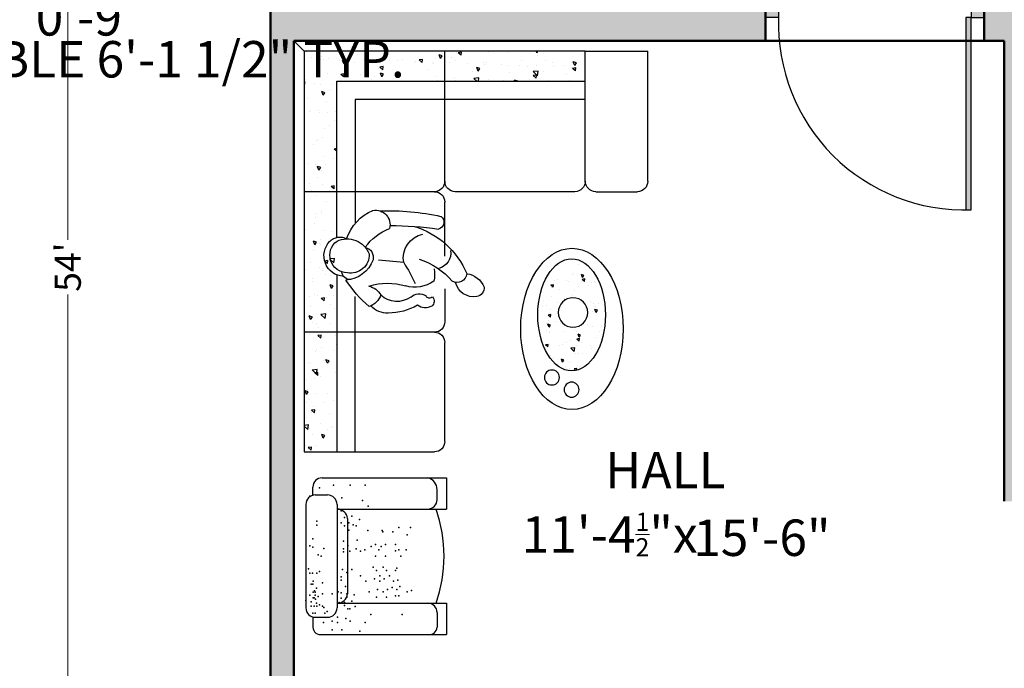
# Model space of a CAD drawing. Units: inches. Extents: x 4508 to 5907, y 877 to 1592.
# Tile 10 of 20: x 5203 to 5392, y 1174 to 1298. Entities that reach past the tile are written whole.
import ezdxf

# ---------------------------------------------------------------- set-up
doc = ezdxf.new("R2010")
doc.units = ezdxf.units.IN
doc.layers.get('DEFPOINTS').update_dxf_attribs({"color": 8})
for name, color, linetype, lineweight in [('A-ANNO-DIMS', 2, 'Continuous', 18), ('A-DOOR', 4, 'Continuous', 25), ('A-FURN', 24, 'Continuous', 18), ('A-WALL', 7, 'Continuous', 50), ('A-WALL-PATT', 8, 'Continuous', 13)]:
    doc.layers.add(name, color=color, linetype=linetype, lineweight=lineweight)
doc.layers.add('doors & windows', color=30, linetype='Continuous')
doc.layers.add('furniture', color=24, linetype='Continuous')
doc.styles.get("Standard").update_dxf_attribs({"font": 'arial.ttf'})
doc.dimstyles.new('details', dxfattribs={"dimtxt": 5, "dimasz": 2, "dimexe": 2, "dimexo": 3, "dimgap": 1, "dimtad": 0, "dimdec": 1, "dimzin": 0, "dimdsep": 46, "dimlunit": 4, "dimtxsty": 'Standard', "dimblk": 'ARCHTICK', "dimcen": 3, "dimclrd": 256, "dimclre": 256, "dimclrt": 256, "dimadec": 0, "dimazin": 0, "dimtfac": 0.5, "dimtdec": 1, "dimtofl": 0, "dimtmove": 0, "dimatfit": 3, "dimldrblk": 'CLOSEDBLANK', "dimfxl": 2, "dimtolj": 1, "dimtzin": 0, "dimlwd": -1, "dimlwe": -1, "dimarcsym": 0})
doc.dimstyles.new('text', dxfattribs={"dimtxt": 7, "dimasz": 0, "dimexe": 3, "dimexo": 3, "dimgap": 0, "dimtad": 1, "dimtih": 1, "dimtoh": 1, "dimzin": 3, "dimdsep": 46, "dimlunit": 4, "dimtxsty": 'Standard', "dimblk": 'CLOSEDBLANK', "dimcen": 3, "dimse1": 1, "dimse2": 1, "dimsd1": 1, "dimsd2": 1, "dimclrd": 256, "dimclre": 256, "dimclrt": 256, "dimadec": 0, "dimazin": 0, "dimtfac": 0.5, "dimtofl": 0, "dimtmove": 0, "dimatfit": 3, "dimfxl": 3, "dimtolj": 1, "dimtzin": 0, "dimlwd": -1, "dimlwe": -1, "dimarcsym": 0})

# ---------------------------------------------------------------- blocks, each defined once
blk = doc.blocks.new('_ArchTick')
at = {"color": 0, "linetype": 'ByBlock', "const_width": 0.15}
blk.add_lwpolyline([(-0.5, -0.5), (0.5, 0.5)], dxfattribs=at)
blk = doc.blocks.new('*D77')
at = {"layer": 'A-ANNO-DIMS', "color": 0, "transparency": 16777216}
for p, q in [((5201.49, 1574.7), (5213.97, 1574.7)), ((5211.97, 1574.7), (5211.97, 1255.95)), ((5211.97, 926.7), (5211.97, 1245.46)), ((5201.49, 926.7), (5213.97, 926.7))]:
    blk.add_line(p, q, dxfattribs=at)
at = {"layer": 'DEFPOINTS', "color": 0, "transparency": 16777216}
for p in [(5198.49, 1574.7), (5211.97, 1574.7), (5198.49, 926.7)]:
    blk.add_point(p, dxfattribs=at)
at = {"layer": 'A-ANNO-DIMS', "color": 0, "transparency": 16777216, "xscale": 2, "yscale": 2, "zscale": 2}
for p, rotation in [((5211.97, 1574.7), 90), ((5211.97, 926.7), 270)]:
    blk.add_blockref('_ArchTick', p, dxfattribs=dict(at, rotation=rotation))
at = {"layer": 'A-ANNO-DIMS', "color": 0, "transparency": 16777216, "insert": (5211.97, 1250.7), "char_height": 5, "attachment_point": 5, "rotation": 90}
blk.add_mtext("\\A1;54'", dxfattribs=at)
blk = doc.blocks.new('_ClosedBlank')
at = {"color": 0, "lineweight": -2}
for p, q in [((-1, 0.167), (0, 0)), ((-1, 0.167), (-1, -0.167)), ((0, 0), (-1, -0.167))]:
    blk.add_line(p, q, dxfattribs=at)
blk = doc.blocks.new('MAN')
at = {"layer": 'doors & windows'}
blk.add_line((1.3, -9.85), (0.89, -5.45), dxfattribs=at)
for centre, radius, start, end in [((0.1, 0.48), 3.6, 2.8928, 134.5528), ((-0.81, 1.3), 2.37, 132.7993, 210.1219), ((1.3, 0.05), 4.16, 155.2349, 248.5051), ((0, 0), 3.06, 359.7942, 144.0351), ((-0.36, -7.56), 8.07, 108.0153, 157.5724), ((-0.98, 0.55), 5.34, 289.2819, 356.6237), ((2.86, -0.44), 1.38, 352.7443, 87.7525), ((-8.99, -19.77), 24.04, 41.647, 56.3067), ((-0.1, -0.61), 3.22, 267.7788, 10.6507), ((4.14, -10.82), 9.46, 125.6851, 158.6987), ((0.38, -2.75), 1.79, 192.3382, 283.0231), ((-5.32, -4.92), 2.54, 170.002, 284.7527), ((15.87, -7.04), 10.97, 162.7002, 196.7262), ((8.59, -3.01), 3.29, 193.5598, 239.9446), ((5.83, -2.73), 3.32, 289.6374, 341.2911), ((6.12, -7.03), 4.01, 358.2671, 46.939), ((34.75, -7.19), 42.53, 177.9613, 192.4551), ((3.84, -8.67), 4.24, 325.4363, 41.8446), ((54.76, -7.35), 59.95, 180.1044, 188.2297), ((-0.78, -6.94), 10.91, 330.7562, 358.8997), ((0.5, -14.05), 4.27, 79.2575, 168.509), ((16.49, 13.41), 27.78, 236.8487, 245.427), ((-0.19, -11.81), 5.78, 325.2412, 16.1794), ((9.03, -7.36), 14.72, 197.1765, 246.7641), ((8.85, -12.54), 2.12, 136.0875, 215.1077), ((12.84, -8.62), 12.77, 197.9012, 229.3504), ((7.06, -13.61), 2.15, 328.4119, 38.6474), ((3.21, -8.72), 6.53, 262.8142, 281.931), ((6.8, -14.37), 0.689, 315.9836, 61.7947), ((8.05, -14.12), 1.05, 224.0636, 323.687), ((-5.78, -15.61), 1.25, 217.214, 345.0614), ((-0.4, -15.27), 2.81, 261.6005, 345.5998), ((3.09, -19.2), 1.68, 274.444, 31.8659), ((4.09, -22.01), 3.16, 349.15, 77.9716), ((6.99, -20.36), 3.8, 187.9766, 248.0432), ((5.75, -22.44), 1.45, 262.6631, 353.5986)]:
    blk.add_arc(centre, radius, start, end, dxfattribs=at)
blk = doc.blocks.new('sofa 3')
at = {"layer": 'furniture', "ltscale": 0.5}
h = blk.add_hatch(dxfattribs=at)
h.set_pattern_fill('AR-CONC', color=256, angle=90, style=0)
h.set_pattern_definition([(220, (1099.1507, -871.655), (0.627521, -7.172602), [0.75, -8.25]), (275, (1099.151, -871.655), (-7.52192, 1.387513), [0.6, -6.6]), (169.5486, (1099.203, -872.253), (-6.894395, -5.785094), [0.637402, -7.01142]), (223.8158, (1097.151, -871.655), (1.65519, -10.67241), [1.125, -12.375]), (173.3644, (1097.289, -872.544), (-9.74118, -9.34663), [0.9561, -10.51713]), (278.8158, (1097.151, -871.655), (-9.74119, -9.34662), [0.9, -9.9]), (249, (1097.6507, -872.655), (4.02619, -5.96907), [0.75, -8.25]), (304, (1097.651, -872.655), (-7.2515, -2.433153), [0.6, -6.6]), (198.5486, (1097.986, -873.1524), (-3.225305, -8.402226), [0.637402, -7.01142]), (232.5, (1099.1507, -871.655), (-3.3289385, -0.1215986), [0, -6.52, 0, -6.7, 0, -6.625]), (262.5, (1099.1507, -871.655), (-3.944117, -2.630695), [0, -3.82, 0, -6.37, 0, -2.525]), (302.5, (1099.1507, -869.425), (0.2255487, -5.3382244), [0, -2.5, 0, -7.8, 0, -10.35]), (312.5, (1099.1507, -868.425), (-1.00105, -5.831862), [0, -3.25, 0, -5.18, 0, -7.35])])
h.paths.add_polyline_path([(2, 56), (2, 79), (8.27, 79), (8.27, 56)])
edge = h.paths.add_edge_path()
edge.add_arc((9.44, 36.7), 1.54, 139.4115, 177.7525)
edge.add_arc((8.94, 33.52), 3.4, 107.8673, 234.0351)
edge.add_arc((8.88, 34.97), 4.62, 245.2349, 262.3616)
edge.add_line((8.27, 30.38), (8.27, 29))
edge.add_line((8.27, 29), (2, 29))
edge.add_line((2, 29), (2, 56))
edge.add_line((2, 56), (8.27, 56))
edge.add_line((8.27, 56), (8.27, 37.7))
h.paths.add_polyline_path([(8.27, 7.77), (29, 7.77), (29, 2), (2, 2), (2, 29), (8.27, 29)])
h.paths.add_polyline_path([(29, 2), (29, 7.77), (56, 7.77), (56, 2)])
at = {"layer": 'furniture'}
h = blk.add_hatch(dxfattribs=at)
h.set_pattern_fill('AR-CONC', color=256, scale=0.8, angle=90, style=0)
h.set_pattern_definition([(220, (892.888, -686.9864), (0.502017, -5.738081), [0.6, -6.6]), (275, (892.888, -686.9864), (-6.017537, 1.11001), [0.48, -5.28]), (169.5486, (892.93, -687.4646), (-5.515516, -4.628075), [0.509922, -5.609137]), (223.8158, (891.288, -686.9864), (1.32415, -8.53793), [0.9, -9.9]), (173.3644, (891.3985, -687.698), (-7.79294, -7.4773), [0.76488, -8.413704]), (278.8158, (891.288, -686.986), (-7.79295, -7.477296), [0.72, -7.92]), (249, (891.688, -687.7864), (3.220951, -4.775256), [0.6, -6.6]), (304, (891.688, -687.7864), (-5.8012, -1.946523), [0.48, -5.28]), (198.5486, (891.9566, -688.1844), (-2.580244, -6.72178), [0.509922, -5.609137]), (232.5, (892.8881, -686.9864), (-2.663151, -0.097279), [0, -5.216, 0, -5.36, 0, -5.3]), (262.5, (892.8881, -686.9864), (-3.155294, -2.104556), [0, -3.056, 0, -5.096, 0, -2.02]), (302.5, (892.8881, -685.2024), (0.180439, -4.2705795), [0, -2, 0, -6.24, 0, -8.28]), (312.5, (892.888, -684.4024), (-0.80084, -4.665489), [0, -2.6, 0, -4.144, 0, -5.88])])
edge = h.paths.add_edge_path()
edge.add_ellipse((53.37, 52.67), major_axis=(0, 10.76), ratio=0.60396, start_angle=0, end_angle=360, ccw=False)
h.paths.add_polyline_path([(56.46, 52.22, -1), (50.81, 52.22, -1)], flags=16)
for p, q in [((2, 2), (2, 79)), ((2, 79), (27, 79)), ((8.27, 44.99), (8.27, 79)), ((11.8, 79), (11.8, 49.12)), ((29, 77), (29, 58)), ((27, 56), (2, 56)), ((29, 47.65), (29, 54)), ((29, 41.41), (29, 31)), ((8.27, 37.77), (8.27, 7.77)), ((11.8, 11.29), (11.8, 35.08)), ((8.27, 29), (2, 29)), ((27, 29), (8.27, 29)), ((54, 29), (31, 29)), ((58, 29), (66, 29)), ((29, 27), (29, 2)), ((56, 27), (56, 2)), ((68, 27), (68, 2)), ((56, 11.29), (11.8, 11.29)), ((8.27, 7.77), (56, 7.77)), ((2, 2), (0, 0)), ((56, 2), (2, 2)), ((56, 2), (68, 2))]:
    blk.add_line(p, q, dxfattribs=at)
for centre, radius in [((53.36, 67.05), 1.44), ((49.58, 64.71), 1.44), ((53.63, 52.22), 2.83)]:
    blk.add_circle(centre, radius, dxfattribs=at)
for centre, start, end in [((27, 77), 0, 90), ((27, 58), 270, 0), ((27, 54), 0, 90), ((27, 31), 270, 0), ((27, 27), 0, 90), ((31, 27), 90, 180), ((54, 27), 0, 90), ((58, 27), 90, 180), ((66, 27), 0, 90)]:
    blk.add_arc(centre, 2, start, end, dxfattribs=at)
at = {"layer": 'furniture', "extrusion": (0, 0, -1)}
for centre, major_axis, ratio in [((53.43, 55.37), (0, 15.49), 0.635514), ((53.37, 52.67), (0, 10.76), 0.60396)]:
    blk.add_ellipse(centre, major_axis=major_axis, ratio=ratio, dxfattribs=at)
at = {"xscale": 1.1, "yscale": 1.1, "zscale": 1.1, "rotation": 90}
blk.add_blockref('MAN', (10.27, 41.21), dxfattribs=at)
blk = doc.blocks.new('MD')
at = {"layer": 'doors & windows'}
h = blk.add_hatch(dxfattribs=at)
h.set_pattern_fill('DOTS', color=256, scale=2, style=0)
h.set_pattern_definition([(180, (0, -4), (-0.0625, 0.125), [0, -0.125])])
h.paths.add_polyline_path([(2.5, 37), (3.5, 37), (3.5, 0), (2.5, 0)])
h = blk.add_hatch(dxfattribs=at)
h.set_pattern_fill('DOTS', color=256, scale=2, style=0)
h.set_pattern_definition([(0, (0, -0.5), (0.0625, 0.125), [0, -0.125])])
h.paths.add_polyline_path([(42, -4.5), (42, 0), (39.5, 0), (39.5, -1.5), (39, -1.5), (39, -3.75), (39.25, -3.75, 0.403966), (39.75, -4.25), (39.75, -4.5)])
h.paths.add_polyline_path([(0, -4.5), (2.25, -4.5), (2.25, -4.25, 0.403966), (2.75, -3.75), (3, -3.75), (3, -1.5), (2.5, -1.5), (2.5, 0), (0, 0)])
for p, q in [((0, 0), (0, -4.5)), ((42, 0), (42, -4.5))]:
    blk.add_line(p, q)
blk.add_line((0, -4.5), (2.25, -4.5), dxfattribs=at)
blk.add_lwpolyline([(3.5, 0), (3.5, 37), (2.5, 37), (2.5, 0)], close=True, dxfattribs=at)
for points in [[(3, -3.75), (3, -1.5), (2.5, -1.5), (2.5, 0), (0, 0)], [(39, -3.75), (39, -1.5), (39.5, -1.5), (39.5, 0), (42, 0)], [(42, -4.5), (39.75, -4.5)]]:
    blk.add_lwpolyline(points, dxfattribs=at)
for points in [[(2.25, -4.5), (2.25, -4.25, 0.403966), (2.75, -3.75), (3, -3.75)], [(39.75, -4.5), (39.75, -4.25, -0.403966), (39.25, -3.75), (39, -3.75)]]:
    blk.add_lwpolyline(points, format="xyb", dxfattribs=at)
at = {"layer": 'doors & windows', "ltscale": 6}
blk.add_arc((3.73, 1.23), 35.79, 358.0281, 91.9719, dxfattribs=at)
at = {"layer": 'doors & windows'}
blk.add_point((21, -2.75), dxfattribs=at)
blk = doc.blocks.new('sofa')
at = {"layer": 'furniture'}
for p, q in [((1.33, 11.75), (1.33, 13.25)), ((3.13, 15.05), (27, 15.05)), ((27, 15.05), (27, 9.05)), ((1.8, 11.75), (4.13, 11.75)), ((25.2, 10.85), (25.2, 12.75)), ((0, 9.95), (0, -9.95)), ((6, 9.95), (6, -9.95)), ((6, 9.05), (27, 9.05)), ((8, 7.25), (8, -7.25)), ((8, 4.04), (8, 3.89)), ((6.03, -9.05), (27, -9.05)), ((27, -9.05), (27, -15.05)), ((25.2, -10.85), (25.2, -13.65)), ((1.33, -11.75), (1.33, -13.65)), ((1.8, -11.75), (4.13, -11.75)), ((3.13, -15.05), (27, -15.05))]:
    blk.add_line(p, q, dxfattribs=at)
for centre, radius, start, end in [((3.13, 13.25), 1.8, 90, 180), ((22.91, 12.82), 2.29, 358.3453, 77.7487), ((1.8, 9.95), 1.8, 90, 180), ((1.8, 9.95), 1.8, 90, 180), ((4.14, 9.89), 1.86, 1.747, 90.2901), ((4.14, 9.89), 1.86, 1.747, 90.2901), ((23.4, 10.85), 1.8, 270, 0), ((5.91, 6.93), 2.12, 8.589, 87.4366), ((-0.79, 0), 27.33, 340.6621, 19.3379), ((5.96, -6.99), 2.06, 272.0036, 352.7589), ((23.4, -10.85), 1.8, 0, 90), ((1.8, -9.95), 1.8, 180, 270), ((4.14, -9.89), 1.86, 269.7099, 358.253), ((2.83, -13.59), 1.5, 182.4941, 281.7559), ((23.7, -13.59), 1.5, 258.2441, 357.5059)]:
    blk.add_arc(centre, radius, start, end, dxfattribs=at)
for p in [(5.3, 13.66), (8.48, 13.66), (11.4, 13.66), (0.72, 11.51), (2.64, 13.13), (6.89, 11.2), (10.87, 10.67), (11.93, 9.61), (6.8, 8.68), (8.85, 7.66), (2.09, 5.95), (2.11, 6.75), (6.8, 6.43), (7.42, 7.45), (7.42, 5.82), (8.24, 6.43), (9.05, 6.02), (9.67, 5.82), (10.28, 7.04), (8.24, 5), (11.92, 4.9), (14.64, 4.9), (14.78, 4.7), (16.69, 4.7), (17.83, 5.52), (19.47, 4.09), (20.08, 5.52), (0.72, 1.97), (1.32, 3.3), (7.21, 2.86), (8.03, 2.04), (9.87, 3.06), (13.35, 2.21), (15.26, 2.21), (17.21, 2.25), (1.3, 1.71), (2.38, 0.24), (3.44, 1.44), (7.21, 1.39), (7.21, 0.82), (8.44, 0.98), (9.67, 1.43), (10.49, 0.98), (11.31, 1.19), (12.53, 1.84), (13.35, 0.01), (14.03, 1.19), (14.44, 1.84), (15.26, 0.01), (17.24, 1.02), (17.85, 1.19), (19.26, 1.19), (2.91, -0.01), (18.24, -0.03), (0.5, -2.45), (0.72, -3.25), (1.26, -3.25), (2.11, -3.25), (2.64, -2.98), (7.01, -2.55), (7.83, -3.16), (8.85, -2.55), (10.49, -3.77), (12.94, -2.14), (13.56, -2.75), (14.17, -3.77), (14.85, -2.14), (15.46, -2.75), (16.07, -3.77), (17.21, -2.75), (17.44, -2.34), (1.03, -5.36), (1.32, -5.36), (1.36, -4.83), (3.17, -5.1), (6.8, -3.98), (6.8, -4.59), (11.51, -4.79), (13.15, -4.38), (14.23, -4.79), (15.05, -4.38), (16.8, -4.79), (17.65, -4.59), (0.77, -7.48), (1.36, -6.95), (1.62, -6.69), (1.79, -6.95), (1.79, -7.48), (2.05, -6.16), (3.17, -7.22), (5.03, -7.22), (6.19, -6.84), (6.8, -7.04), (7.62, -5.82), (7.83, -7.25), (9.26, -7.45), (12.12, -6.84), (13.76, -6.43), (14.85, -6.84), (15.66, -6.43), (16.6, -6.02), (17.44, -6.43), (18.06, -5.82), (19.47, -6.84), (20.28, -6.63), (-0.03, -8.54), (1.03, -8.81), (1.36, -8.01), (1.56, -8.01), (1.85, -8.28), (2.05, -9.07), (2.38, -7.75), (2.64, -9.34), (6.39, -8.88), (6.8, -8.06), (7.42, -8.88), (7.83, -7.86), (8.85, -8.68), (13.56, -7.86), (15.46, -7.86), (17.24, -7.65), (17.83, -7.65), (0.99, -9.6), (1.3, -10.93), (1.58, -9.6), (1.79, -10.93), (2.09, -9.6), (3.17, -9.6), (3.44, -9.87), (3.64, -10.93), (4.09, -10.66), (7.42, -9.49), (8.03, -10.11), (8.44, -10.11), (9.46, -9.7), (12.46, -11.19), (18.51, -11.19), (3.38, -12.78), (5.03, -12.52), (6.09, -11.72), (6.09, -12.78), (7.69, -11.99), (8.48, -12.52), (11.4, -12.78), (5.03, -14.17), (6.89, -14.17), (10.34, -14.44)]:
    blk.add_point(p, dxfattribs=at)
blk = doc.blocks.new('*D98')
at = {"layer": 'DEFPOINTS', "color": 0, "transparency": 16777216}
for p in [(5255.4, 1205.15), (5391.9, 1205.7), (5255.4, 1203.74)]:
    blk.add_point(p, dxfattribs=at)
at = {"layer": 'A-ANNO-DIMS', "color": 0, "transparency": 16777216, "insert": (5316.09, 1205.15), "char_height": 7, "attachment_point": 5}
blk.add_mtext('\\A1;          HALL\\P11\'-4{\\H0.5x;\\S1/2;}"x', dxfattribs=at)
blk = doc.blocks.new('*D99')
at = {"layer": 'DEFPOINTS', "color": 0, "transparency": 16777216}
for p in [(5336.4, 1294.2), (5345.32, 1294.2), (5334.11, 1108.2)]:
    blk.add_point(p, dxfattribs=at)
at = {"layer": 'A-ANNO-DIMS', "color": 0, "transparency": 16777216, "insert": (5345.32, 1198.7), "char_height": 7, "attachment_point": 5}
blk.add_mtext('\\A1;15\'-6"', dxfattribs=at)
blk = doc.blocks.new('*D172')
at = {"layer": 'DEFPOINTS', "color": 0, "transparency": 16777216}
for p in [(5076.25, 1287.03), (5076.25, 1276.01), (5149.75, 1276.01)]:
    blk.add_point(p, dxfattribs=at)
at = {"layer": 'A-ANNO-DIMS', "transparency": 16777216, "insert": (5214.38, 1290.65), "char_height": 7, "attachment_point": 5}
blk.add_mtext('\\A1;DINING TABLE 6\'-1 1/2" TYP.', dxfattribs=at)
blk = doc.blocks.new('*D188')
at = {"layer": 'DEFPOINTS', "color": 0, "transparency": 16777216}
for p in [(5259.90304, 1303.203772), (5216.35304, 1294.203772), (5255.40304, 1294.203772)]:
    blk.add_point(p, dxfattribs=at)
at = {"layer": 'A-ANNO-DIMS', "transparency": 16777216, "insert": (5216.35304, 1298.703772), "char_height": 7, "attachment_point": 5}
blk.add_mtext('\\A1;0\'-9"', dxfattribs=at)

msp = doc.modelspace()

# ---------------------------------------------------------------- hatches: boundary and pattern name
at = {"layer": 'A-WALL-PATT'}
h = msp.add_hatch(color=256, dxfattribs=at)
h.dxf.hatch_style = 1
h.paths.add_polyline_path([(5529.903, 1303.204), (5388.02, 1303.204), (5388.02, 1294.204), (5391.903, 1294.204), (5391.903, 1205.704), (5396.403, 1205.704), (5396.403, 1294.204), (5489.403, 1294.204), (5489.403, 1256.139), (5493.903, 1256.139), (5493.903, 1294.204), (5529.903, 1294.204)], flags=17)
h.paths.add_polyline_path([(5346.02, 1303.204), (5322.903, 1303.204), (5322.903, 1321.388), (5313.903, 1321.388), (5313.903, 1303.204), (5259.903, 1303.204), (5259.903, 1381.204), (5313.903, 1381.204), (5313.903, 1359.674), (5322.903, 1359.674), (5322.903, 1381.204), (5338.979, 1381.204), (5338.979, 1390.204), (5331.903, 1390.204), (5331.903, 1442.704), (5255.403, 1442.704), (5255.403, 1570.204), (5387.403, 1570.204), (5387.403, 1541.271), (5391.903, 1541.271), (5391.903, 1570.204), (5483.403, 1570.204), (5483.403, 1498.204), (5391.903, 1498.204), (5391.903, 1509.559), (5387.403, 1509.559), (5387.403, 1390.204), (5380.979, 1390.204), (5380.979, 1381.204), (5387.403, 1381.204), (5529.903, 1381.204), (5529.903, 1498.204), (5487.903, 1498.204), (5487.903, 1570.204), (5529.903, 1570.204), (5529.903, 1574.704), (5250.903, 1574.704), (5250.903, 991.204), (5310.903, 991.204), (5310.903, 926.704), (5529.903, 926.704), (5529.903, 1210.204), (5525.403, 1210.204), (5525.403, 1103.704), (5499.903, 1103.704), (5499.903, 1210.204), (5493.903, 1210.204), (5493.903, 1256.139), (5489.403, 1256.139), (5489.403, 1210.204), (5461.584, 1210.204), (5461.584, 1205.704), (5495.403, 1205.704), (5495.403, 1103.704), (5436.903, 1103.704), (5436.903, 1051.204), (5391.954, 1051.204), (5391.954, 1103.03), (5391.954, 1107.53), (5255.403, 1108.204), (5255.403, 1294.204), (5346.02, 1294.204)])
h.paths.add_polyline_path([(5255.403, 1390.204), (5255.403, 1398.204), (5255.403, 1438.204), (5257.903, 1438.204), (5258.903, 1438.204), (5327.403, 1438.204), (5327.403, 1390.204), (5325.903, 1390.204)], flags=16)
h.paths.add_polyline_path([(5288.757, 1390.704), (5288.757, 1390.204), (5292.173, 1390.204), (5292.173, 1390.704)], flags=0)
h.paths.add_polyline_path([(5289.965, 1391.606), (5289.965, 1396.645), (5289.903, 1396.645), (5289.903, 1397.319), (5288.849, 1398.862), (5288.849, 1398.8), (5288.983, 1398.748), (5288.983, 1399.204), (5289.091, 1399.204), (5292.081, 1399.204), (5292.081, 1398.665), (5291.946, 1398.665), (5291.027, 1397.319), (5291.027, 1396.645), (5290.965, 1396.645), (5290.965, 1391.606)], flags=0)
h.paths.add_polyline_path([(5288.849, 1399.069, 2.6374395), (5289.056, 1398.835), (5289.117, 1399.087, 0.9346155)], flags=0)
h.paths.add_polyline_path([(5290.061, 1398.665), (5290.061, 1399.204), (5290.038, 1398.975)], flags=0)
h.paths.add_polyline_path([(5291.946, 1398.934, -1), (5291.946, 1398.665)], flags=0)
h.paths.add_polyline_path([(5289.414, 1398.967), (5289.414, 1399.204), (5289.63, 1399.204), (5289.63, 1398.363), (5290.051, 1397.184), (5290.76, 1397.184), (5290.869, 1398.665), (5290.869, 1399.204), (5290.815, 1398.665), (5290.815, 1399.204), (5291.462, 1399.204), (5291.462, 1398.816), (5290.879, 1397.184), (5290.051, 1397.184)], flags=0)
h.paths.add_polyline_path([(5273.903, 1392.056), (5269.591, 1392.056, 0.0901028), (5265.544, 1392.842), (5265.511, 1392.034, -0.3516542), (5265.903, 1391.546, -1), (5264.903, 1391.546, -0.3042165), (5265.213, 1392.008), (5265.167, 1392.84, 0.0880132), (5261.215, 1392.056), (5256.903, 1392.056), (5256.903, 1398.704, -0.4142136), (5259.403, 1401.204), (5271.403, 1401.204, -0.4142136), (5273.903, 1398.704)], flags=0)
h.paths.add_polyline_path([(5263.726, 1395.073, -1), (5267.08, 1395.073, -1)], flags=0)
h.paths.add_polyline_path([(5264.434, 1395.073, -0.695521), (5265.153, 1395.073, -1.1408699), (5265.403, 1395.585, -0.7522125), (5265.403, 1396.25, 0.3674806)], flags=0)
h.paths.add_polyline_path([(5265.153, 1394.399, -1), (5265.653, 1394.399, -1)], flags=0)
h.paths.add_polyline_path([(5265.905, 1395.077, -1), (5266.405, 1395.077, -1)], flags=0)
h.paths.add_polyline_path([(5307.994, 1403.113, -1), (5307.994, 1417.295), (5318.794, 1417.295, -0.4142136), (5319.794, 1416.295), (5320.794, 1416.295, -0.4142136), (5321.794, 1417.295), (5324.903, 1417.295, -0.4142136), (5325.903, 1416.295), (5325.903, 1404.113, -0.4142136), (5324.903, 1403.113), (5321.794, 1403.113, -0.4142136), (5320.794, 1404.113), (5319.794, 1404.113, -0.4142136), (5318.794, 1403.113)], flags=0)
h.paths.add_polyline_path([(5307.836, 1405.113, -1), (5307.836, 1415.295), (5315.591, 1415.295, -0.4142136), (5317.532, 1413.353), (5317.532, 1407.054, -0.4142136), (5315.591, 1405.113)], flags=0)
h.paths.add_polyline_path([(5312.032, 1408.204, -1), (5312.032, 1412.204), (5315.032, 1412.204, -0.4142136), (5316.032, 1411.204), (5316.032, 1409.204, -0.4142136), (5315.032, 1408.204)], flags=0)
h.paths.add_polyline_path([(5391.903, 1385.704), (5391.903, 1493.704), (5525.403, 1493.704), (5525.403, 1385.704)], flags=16)
h.paths.add_polyline_path([(5422.641, 1390.704), (5422.641, 1465.704, -0.9426302), (5422.641, 1467.704), (5494.547, 1467.704, -1), (5494.665, 1465.704), (5494.665, 1390.704, -0.9426302), (5494.665, 1388.704), (5422.759, 1388.704, -1)], flags=0)
h.paths.add_polyline_path([(5427.52, 1395.749, -0.0238564), (5427.614, 1403.949, 0.0884332), (5427.476, 1405.056, 0.0506693), (5427.273, 1405.463, -0.8716827), (5427.713, 1405.835, 0.0268855), (5431.815, 1405.361, 0.0306964), (5436.289, 1405.361, -0.0263641), (5445.798, 1405.259, 0.075811), (5450.408, 1405.53, 0.0687062), (5454.457, 1405.903, -1.0086747), (5454.781, 1405.482, 0.0692081), (5454.389, 1400.959, -0.0519468), (5454.356, 1394.996, 0.1195012), (5454.627, 1392.895, 0.0143508), (5454.796, 1392.489, -0.6962059), (5454.42, 1392.118, 0.1574808), (5448.747, 1392.794, -0.025536), (5432.749, 1392.774, 0.0920085), (5427.781, 1392.048, -0.9384848), (5427.137, 1392.455, 0.0063894), (5427.314, 1392.79, 0.0472995)], flags=0)
h.paths.add_polyline_path([(5426.125, 1411.372, 0.0617649), (5428.641, 1412.201), (5428.641, 1465.704), (5488.665, 1465.704), (5488.665, 1412.363, 0.2363822), (5467.6, 1412.052, -0.2252042)], flags=0)
h.paths.add_polyline_path([(5391.903, 1490.204), (5391.903, 1491.204), (5422.903, 1491.204), (5422.903, 1490.204)], flags=0)
h.paths.add_polyline_path([(5462.545, 1392.771, 0.1270318), (5462.866, 1394.996, -0.0519468), (5462.832, 1400.959, 0.0692081), (5462.441, 1405.482, -1.0086747), (5462.765, 1405.903, 0.0857004), (5471.424, 1405.259, -0.0263641), (5480.932, 1405.361, 0.0306964), (5485.407, 1405.361, 0.0268855), (5489.509, 1405.835, -0.8716827), (5489.949, 1405.463, 0.0506693), (5489.746, 1405.056, 0.0884332), (5489.608, 1403.949, -0.0238564), (5489.702, 1395.749, 0.0472995), (5489.908, 1392.79, 0.0063894), (5490.085, 1392.455, -0.9384848), (5489.441, 1392.048, 0.0920085), (5484.473, 1392.774, -0.025536), (5468.475, 1392.794, 0.1574808), (5462.802, 1392.118, -0.6962059), (5462.426, 1392.489, 0.0100173), (5462.546, 1392.771)], flags=0)
h.paths.add_polyline_path([(5387.454, 1103.03), (5387.454, 1100.53), (5387.454, 1099.53), (5387.454, 995.03), (5387.454, 991.204), (5391.954, 991.204), (5391.954, 1046.704), (5525.403, 1046.704), (5525.403, 931.182), (5391.954, 930.53), (5391.954, 960.53), (5387.454, 960.53), (5387.454, 930.53), (5315.403, 930.53), (5315.403, 991.204), (5323.403, 991.204), (5387.454, 991.204), (5387.454, 995.03), (5255.403, 995.704), (5255.403, 1103.704)], flags=16)
h.paths.add_polyline_path([(5379.264, 1062.889), (5379.264, 1060.156), (5385.764, 1061.889, -0.4526903), (5385.764, 1059.889), (5379.264, 1059.889), (5379.264, 1055.156), (5385.764, 1056.889, -0.4526903), (5385.764, 1054.889), (5379.264, 1054.889), (5379.264, 1050.156), (5385.764, 1051.889, -0.4526903), (5385.764, 1049.889), (5379.264, 1049.889), (5379.264, 1010.156), (5385.764, 1011.889, -0.4526903), (5385.764, 1009.889), (5379.264, 1009.889), (5379.264, 1005.156), (5385.764, 1006.889, -0.4526903), (5385.764, 1004.889), (5379.264, 1004.889), (5379.264, 1000.156), (5385.764, 1001.889, -0.4526903), (5385.764, 999.889), (5378.264, 999.889), (5370.764, 997.889, -0.6674863), (5370.764, 999.889), (5377.264, 999.889), (5377.264, 1004.623), (5370.764, 1002.889, -0.6674863), (5370.764, 1004.889), (5377.264, 1004.889), (5377.264, 1009.623), (5370.764, 1007.889, -0.6674863), (5370.764, 1009.889), (5377.264, 1009.889), (5377.264, 1049.623), (5370.764, 1047.889, -0.6674863), (5370.764, 1049.889), (5377.264, 1049.889), (5377.264, 1054.623), (5370.764, 1052.889, -0.6674863), (5370.764, 1054.889), (5377.264, 1054.889), (5377.264, 1059.623), (5370.764, 1057.889, -0.6674863), (5370.764, 1059.889), (5377.264, 1059.889), (5377.264, 1062.889)], flags=0)
h.paths.add_polyline_path([(5287.641, 1000.704), (5359.665, 1000.704), (5359.665, 1018.212, 0.3202856), (5332.6, 1022.052, -0.246494), (5287.641, 1023.128)], flags=0)
h.paths.add_polyline_path([(5359.547, 1077.704, -1), (5359.665, 1075.704), (5353.665, 1075.704), (5353.665, 1063.704), (5293.641, 1063.704), (5293.641, 1075.704), (5287.759, 1075.704, -1), (5287.641, 1077.704)], flags=0)
h.paths.add_polyline_path([(5441.403, 1099.204), (5525.403, 1099.204), (5525.403, 1051.204), (5441.403, 1051.204), (5441.403, 1059.204)], flags=16)
h.paths.add_polyline_path([(5441.403, 1096.704), (5466.403, 1096.704), (5466.403, 1095.704), (5441.403, 1095.704)], flags=0)
h.paths.add_polyline_path([(5445.403, 1062.204), (5457.403, 1062.204, -0.4142136), (5459.903, 1059.704), (5459.903, 1053.056), (5455.591, 1053.056, 0.0901028), (5451.544, 1053.842), (5451.511, 1053.034, -0.3516542), (5451.903, 1052.546, -1), (5450.903, 1052.546, -0.3042165), (5451.213, 1053.008), (5451.167, 1053.84, 0.0880132), (5447.215, 1053.056), (5442.903, 1053.056), (5442.903, 1059.704, -0.4142136)], flags=0)
h.paths.add_polyline_path([(5453.08, 1056.073, -1), (5449.726, 1056.073, -1)], flags=0)
h.paths.add_polyline_path([(5292.713, 1015.835, 0.0268855), (5296.815, 1015.361, 0.0306964), (5301.289, 1015.361, -0.0263641), (5310.798, 1015.259, 0.075811), (5315.408, 1015.53, 0.0687062), (5319.457, 1015.903, -1.0086747), (5319.781, 1015.482, 0.0692081), (5319.389, 1010.959, -0.0519468), (5319.356, 1004.996, 0.1195012), (5319.627, 1002.895, 0.0143508), (5319.796, 1002.489, -0.6962059), (5319.42, 1002.118, 0.1574808), (5313.747, 1002.794, -0.025536), (5297.749, 1002.774, 0.0920085), (5292.781, 1002.048, -0.9384848), (5292.137, 1002.455, 0.0063894), (5292.314, 1002.79, 0.0472995), (5292.52, 1005.749, -0.0238564), (5292.614, 1013.949, 0.0884332), (5292.476, 1015.056, 0.0506693), (5292.273, 1015.463, -0.8716827)], flags=0)
h.paths.add_polyline_path([(5450.434, 1056.073, -0.695521), (5451.153, 1056.073, -1.1408699), (5451.403, 1056.585, -0.7522125), (5451.403, 1057.25, 0.3674806)], flags=0)
h.paths.add_polyline_path([(5327.765, 1015.903, 0.0857004), (5336.424, 1015.259, -0.0263641), (5345.932, 1015.361, 0.0306964), (5350.407, 1015.361, 0.0268855), (5354.509, 1015.835, -0.8716827), (5354.949, 1015.463, 0.0506693), (5354.746, 1015.056, 0.0884332), (5354.608, 1013.949, -0.0238564), (5354.702, 1005.749, 0.0472995), (5354.908, 1002.79, 0.0063894), (5355.085, 1002.455, -0.9384848), (5354.441, 1002.048, 0.0920085), (5349.473, 1002.774, -0.025536), (5333.475, 1002.794, 0.1574808), (5327.802, 1002.118, -0.6962059), (5327.426, 1002.489, 0.0100173), (5327.546, 1002.771), (5327.545, 1002.771, 0.1270318), (5327.866, 1004.996, -0.0519468), (5327.832, 1010.959, 0.0692081), (5327.441, 1015.482, -1.0086747)], flags=0)
h.paths.add_polyline_path([(5452.405, 1056.077, -1), (5451.905, 1056.077, -1)], flags=0)
h.paths.add_polyline_path([(5451.653, 1055.399, -1), (5451.153, 1055.399, -1)], flags=0)
h.paths.add_polyline_path([(5472.958, 1051.704), (5472.958, 1051.204), (5476.374, 1051.204), (5476.374, 1051.704)], flags=0)
h.paths.add_polyline_path([(5476.282, 1060.204), (5476.282, 1059.665), (5476.147, 1059.665), (5475.228, 1058.319), (5475.228, 1057.645), (5475.166, 1052.606), (5474.166, 1052.606), (5474.166, 1057.645), (5474.104, 1057.645), (5474.104, 1058.319), (5473.05, 1059.862), (5473.05, 1059.8), (5473.184, 1059.748), (5473.184, 1060.204), (5473.292, 1060.204)], flags=0)
h.paths.add_polyline_path([(5473.05, 1060.069, 2.6374395), (5473.257, 1059.835), (5473.318, 1060.087, 0.9346155)], flags=0)
h.paths.add_polyline_path([(5473.831, 1060.204), (5473.831, 1059.363), (5474.252, 1058.184), (5474.371, 1058.184), (5474.262, 1059.665), (5474.262, 1060.204)], flags=0)
h.paths.add_polyline_path([(5475.501, 1060.204), (5475.501, 1059.363), (5475.555, 1059.514), (5475.555, 1060.204)], flags=0)
h.paths.add_polyline_path([(5474.855, 1060.204), (5474.908, 1060.127), (5474.908, 1060.204), (5474.855, 1059.665)], flags=0)
h.paths.add_polyline_path([(5476.147, 1059.934, -1), (5476.147, 1059.665)], flags=0)
h.paths.add_polyline_path([(5474.693, 1060.204), (5475.178, 1059.511), (5475.178, 1060.204), (5475.285, 1059.934), (5475.285, 1060.204), (5475.178, 1059.665), (5475.178, 1060.204), (5475.07, 1059.665), (5475.07, 1060.204), (5474.962, 1059.665), (5474.962, 1060.204), (5474.693, 1059.306)], flags=0)
h.paths.add_polyline_path([(5474.747, 1060.204), (5474.37, 1059.45), (5474.37, 1060.204), (5474.424, 1060.096), (5474.424, 1060.204), (5474.747, 1059.665)], flags=0)
h.paths.add_polyline_path([(5476.04, 1059.665), (5476.04, 1060.204), (5476.094, 1059.665), (5476.094, 1060.204)], flags=0)
h.paths.add_polyline_path([(5505.994, 1082.295), (5516.794, 1082.295, -0.4142136), (5517.794, 1081.295), (5518.794, 1081.295, -0.4142136), (5519.794, 1082.295), (5522.903, 1082.295, -0.4142136), (5523.903, 1081.295), (5523.903, 1069.113, -0.4142136), (5522.903, 1068.113), (5519.794, 1068.113, -0.4142136), (5518.794, 1069.113), (5517.794, 1069.113, -0.4142136), (5516.794, 1068.113), (5505.994, 1068.113, -1)], flags=0)
h.paths.add_polyline_path([(5505.836, 1080.295), (5513.591, 1080.295, -0.4142136), (5515.532, 1078.353), (5515.532, 1072.054, -0.4142136), (5513.591, 1070.113), (5505.836, 1070.113, -1)], flags=0)
h.paths.add_polyline_path([(5520.403, 963.695), (5520.403, 1035.72), (5502.895, 1035.72, 0.3202856), (5499.055, 1008.654, -0.246494), (5497.978, 963.695)], flags=0)
h.paths.add_polyline_path([(5445.403, 1035.72), (5445.403, 1029.72), (5457.403, 1029.72), (5457.403, 969.695), (5445.403, 969.695), (5445.403, 963.814, -1), (5443.403, 963.695), (5443.403, 1035.602, -1)], flags=0)
h.paths.add_polyline_path([(5510.032, 1077.204), (5513.032, 1077.204, -0.4142136), (5514.032, 1076.204), (5514.032, 1074.204, -0.4142136), (5513.032, 1073.204), (5510.032, 1073.204, -1)], flags=0)
h.paths.add_polyline_path([(5317.255, 989.704), (5323.903, 989.704, -0.4142136), (5326.403, 987.204), (5326.403, 975.204, -0.4142136), (5323.903, 972.704), (5317.255, 972.704), (5317.255, 977.016, 0.0901028), (5318.041, 981.063), (5317.233, 981.096, -0.8964437), (5316.245, 981.204, -0.8220123), (5317.207, 981.394), (5318.04, 981.44, 0.0880132), (5317.255, 985.392)], flags=0)
h.paths.add_polyline_path([(5321.949, 981.204, -1), (5318.594, 981.204, -1)], flags=0)
h.paths.add_polyline_path([(5362.454, 988.03), (5387.454, 988.03), (5387.454, 990.53), (5391.954, 990.53), (5391.704, 988.289, -0.4090807), (5391.204, 987.78), (5391.204, 987.53), (5388.954, 987.53), (5388.954, 988.03), (5387.454, 988.03), (5387.454, 987.03), (5362.474, 987.03, 0.4025427), (5387.454, 963.03), (5388.954, 963.03), (5388.954, 963.53), (5391.195, 963.28, -0.4142136), (5391.704, 962.771), (5391.954, 960.53), (5391.954, 962.78), (5391.704, 962.78, 0.4090807), (5391.195, 963.28), (5388.954, 963.53), (5388.954, 963.03), (5387.454, 963.03, -0.4025427), (5362.474, 987.03), (5362.454, 987.03)], flags=0)
h.paths.add_polyline_path([(5321.285, 981.204, -0.6555366), (5320.522, 981.204, -1.1195284), (5320.275, 980.701, -1.3500746), (5320.279, 980.026, 0.3749463)], flags=0)
h.paths.add_polyline_path([(5320.022, 981.923, -1), (5320.522, 981.923, -1)], flags=0)
h.paths.add_polyline_path([(5319.348, 981.204, -1), (5319.848, 981.204, -1)], flags=0)
h.paths.add_polyline_path([(5507.157, 1030.662, -0.0238564), (5515.358, 1030.756, 0.0472995), (5518.317, 1030.962, 0.0063894), (5518.652, 1031.139, -0.9384848), (5519.059, 1030.495, 0.0920085), (5518.333, 1025.527, -0.025536), (5518.313, 1009.53, 0.1574808), (5518.989, 1003.857, -0.6962059), (5518.618, 1003.48, 0.0100173), (5518.335, 1003.601), (5518.335, 1003.6, 0.1270318), (5516.111, 1003.921, -0.0519468), (5510.148, 1003.887, 0.0692081), (5505.624, 1003.495, -1.0086747), (5505.204, 1003.819, 0.0857004), (5505.848, 1012.479, -0.0263641), (5505.746, 1021.987, 0.0306964), (5505.746, 1026.462, 0.0268855), (5505.272, 1030.563, -0.8716827), (5505.644, 1031.004, 0.0506693), (5506.051, 1030.801, 0.0884332)], flags=0)
h.paths.add_polyline_path([(5368.045, 945.621), (5378.845, 945.621, -0.4142136), (5379.845, 944.621), (5380.845, 944.621, -0.4142136), (5381.845, 945.621), (5384.954, 945.621, -0.4142136), (5385.954, 944.621), (5385.954, 932.439, -0.4142136), (5384.954, 931.439), (5381.845, 931.439, -0.4142136), (5380.845, 932.439), (5379.845, 932.439, -0.4142136), (5378.845, 931.439), (5368.045, 931.439, -1)], flags=0)
h.paths.add_polyline_path([(5327.31, 931.03), (5327.31, 930.53), (5330.726, 930.53), (5330.726, 931.03)], flags=0)
h.paths.add_polyline_path([(5330.634, 939.53), (5330.634, 938.991), (5330.499, 938.991), (5329.579, 937.645), (5329.579, 936.971), (5329.518, 936.971), (5329.518, 931.933), (5328.518, 931.933), (5328.518, 936.971), (5328.456, 936.971), (5328.456, 937.645), (5327.402, 939.189), (5327.402, 939.126), (5327.536, 939.074), (5327.536, 939.53), (5327.644, 939.53)], flags=0)
h.paths.add_polyline_path([(5327.402, 939.395, 2.6374395), (5327.609, 939.161), (5327.67, 939.414, 0.9346155)], flags=0)
h.paths.add_polyline_path([(5328.021, 939.142), (5328.021, 939.53), (5327.967, 939.53), (5327.967, 939.293)], flags=0)
h.paths.add_polyline_path([(5328.614, 939.53), (5328.614, 938.991), (5328.723, 937.51), (5329.313, 937.51), (5329.422, 938.991), (5329.422, 939.53), (5329.368, 938.991), (5329.368, 939.53)], flags=0)
h.paths.add_polyline_path([(5329.853, 939.53), (5329.853, 938.689), (5329.907, 938.84), (5329.907, 939.53)], flags=0)
h.paths.add_polyline_path([(5330.499, 939.261, -1), (5330.499, 938.991)], flags=0)
h.paths.add_polyline_path([(5367.887, 943.621), (5375.641, 943.621, -0.4142136), (5377.583, 941.68), (5377.583, 935.38, -0.4142136), (5375.641, 933.439), (5367.887, 933.439, -1)], flags=0)
h.paths.add_polyline_path([(5509.267, 947.14), (5509.267, 939.64), (5511.267, 932.14, -0.4526903), (5509.267, 932.14), (5509.267, 938.64), (5504.534, 938.64), (5506.267, 932.14, -0.4526903), (5504.267, 932.14), (5504.267, 938.64), (5499.534, 938.64), (5501.267, 932.14, -0.4526903), (5499.267, 932.14), (5499.267, 938.64), (5459.534, 938.64), (5461.267, 932.14, -0.4526903), (5459.267, 932.14), (5459.267, 938.64), (5454.534, 938.64), (5456.267, 932.14, -0.4526903), (5454.267, 932.14), (5454.267, 938.64), (5449.534, 938.64), (5451.267, 932.14, -0.4526903), (5449.267, 932.14), (5449.267, 939.64), (5447.267, 947.14, -0.3030853), (5448.267, 947.808), (5508.266, 947.808, -0.3032033)], flags=0)
h.paths.add_polyline_path([(5510.148, 995.444, -0.0519468), (5516.111, 995.41, 0.1195012), (5518.212, 995.681, 0.0143508), (5518.618, 995.851, -0.6962059), (5518.989, 995.474, 0.1574808), (5518.313, 989.801, -0.025536), (5518.333, 973.804, 0.0920085), (5519.059, 968.836, -0.9384848), (5518.652, 968.192, 0.0063894), (5518.317, 968.369, 0.0472995), (5515.358, 968.575, -0.0238564), (5507.157, 968.669, 0.0884332), (5506.051, 968.531, 0.0506693), (5505.644, 968.327, -0.8716827), (5505.272, 968.768, 0.0268855), (5505.746, 972.869, 0.0306964), (5505.746, 977.344, -0.0263641), (5505.848, 986.852, 0.075811), (5505.576, 991.462, 0.0687062), (5505.204, 995.512, -1.0086747), (5505.624, 995.836, 0.0692081)], flags=0)
h.paths.add_polyline_path([(5372.083, 940.53), (5375.083, 940.53, -0.4142136), (5376.083, 939.53), (5376.083, 937.53, -0.4142136), (5375.083, 936.53), (5372.083, 936.53, -1)], flags=0)
h.paths.add_polyline_path([(5409.258, 1465.643), (5487.738, 1465.643), (5487.738, 1492.394), (5409.258, 1492.394)], flags=8)
h.paths.add_polyline_path([(5463.574, 1465.103), (5486.546, 1465.103), (5486.546, 1479.528), (5463.574, 1479.528)], flags=8)
h.paths.add_polyline_path([(5248.665, 1406.171), (5299.981, 1406.171), (5299.981, 1432.34), (5248.665, 1432.34)], flags=9)
h.paths.add_polyline_path([(5287.471, 1405.121), (5310.443, 1405.121), (5310.443, 1419.546), (5287.471, 1419.546)], flags=8)
h.paths.add_polyline_path([(5371.637, 1047.927), (5371.637, 1010.764), (5377.841, 1010.764), (5377.841, 1047.927)], flags=8)
h.paths.add_polyline_path([(5324.882, 1074.869), (5347.854, 1074.869), (5347.854, 1089.294), (5324.882, 1089.294)], flags=8)
h.paths.add_polyline_path([(5262.863, 1074.665), (5351.123, 1074.665), (5351.123, 1100.833), (5262.863, 1100.833)], flags=8)
h.paths.add_polyline_path([(5307.238, 938.814), (5363.988, 938.814), (5363.988, 964.982), (5307.238, 964.982)], flags=24)
h.paths.add_polyline_path([(5348.837, 937.997), (5371.809, 937.997), (5371.809, 952.422), (5348.837, 952.422)], flags=8)
h.paths.add_polyline_path([(5432.497, 1066.695), (5489.247, 1066.695), (5489.247, 1092.863), (5432.497, 1092.863)], flags=24)
h.paths.add_polyline_path([(5473.52, 1065.943), (5496.492, 1065.943), (5496.492, 1080.368), (5473.52, 1080.368)], flags=8)
h.paths.add_polyline_path([(5451.783, 984.266), (5480.194, 984.266), (5480.194, 998.691), (5451.783, 998.691)], flags=8)
h.paths.add_polyline_path([(5392.211, 983.632), (5481.554, 983.632), (5481.554, 1010.383), (5392.211, 1010.383)], flags=8)
h.paths.add_polyline_path([(5497.304, 946.267), (5460.142, 946.267), (5460.142, 940.062), (5497.304, 940.062)], flags=8)

# ---------------------------------------------------------------- linework, layer by layer
at = {"layer": 'A-WALL'}
for p, q in [((5250.903, 926.704), (5250.903, 1574.704)), ((5346.02, 1303.204), (5346.02, 1294.204)), ((5388.02, 1303.204), (5388.02, 1294.204)), ((5255.403, 1294.204), (5391.903, 1294.204)), ((5255.403, 1108.204), (5255.403, 1294.204)), ((5391.903, 1294.204), (5391.903, 1205.704))]:
    msp.add_line(p, q, dxfattribs=at)

# ---------------------------------------------------------------- block references
at = {"layer": 'A-DOOR', "rotation": 180}
msp.add_blockref('MD', (5388.02, 1298.704), dxfattribs=at)
at = {"layer": 'A-FURN', "xscale": -1, "rotation": 180}
msp.add_blockref('sofa 3', (5255.403, 1294.204), dxfattribs=at)
at = {"layer": 'A-FURN'}
msp.add_blockref('sofa', (5257.72, 1195.163), dxfattribs=at)

# ---------------------------------------------------------------- dimensions: what is measured, and where the dimension line sits
at = {"layer": 'A-ANNO-DIMS'}
for base, p1, p2, dimstyle, override, picture, middle in [((5211.971, 1574.704), (5198.492, 926.704), (5198.492, 1574.704), 'details', {"dimclrd": 0, "dimclre": 0, "dimclrt": 0}, '*D77', (5211.971, 1250.704)), ((5216.353, 1294.204), (5259.903, 1303.204), (5255.403, 1294.204), 'text', {"dimdec": 1, "dimlfac": 1, "dimrnd": 0, "dimzin": 1, "dimdsep": 46, "dimlunit": 4, "dimfrac": 2}, '*D188', (5216.353, 1298.704))]:
    dim = msp.add_linear_dim(base=base, p1=p1, p2=p2, angle=90, dimstyle=dimstyle, override=override, dxfattribs=at)
    dim.commit()
    dim.dimension.update_dxf_attribs({"geometry": picture, "text_midpoint": middle})
dim = msp.add_linear_dim(base=(5076.246, 1287.034), p1=(5149.746, 1276.009), p2=(5076.246, 1276.009), angle=180, text='DINING TABLE <> TYP.', dimstyle='text', override={"dimdec": 1, "dimrnd": 0, "dimzin": 1, "dimlunit": 4, "dimfrac": 2}, dxfattribs=at)
dim.commit()
dim.dimension.update_dxf_attribs({"geometry": '*D172', "text_midpoint": (5214.381, 1290.653)})
dim = msp.add_linear_dim(base=(5345.321, 1294.204), p1=(5334.11, 1108.204), p2=(5336.404, 1294.204), angle=90, dimstyle='text', override={"dimclrd": 0, "dimclre": 0, "dimclrt": 0}, dxfattribs=at)
dim.commit()
dim.dimension.update_dxf_attribs({"geometry": '*D99', "text_midpoint": (5345.321, 1198.701), "dimtype": 160})
dim = msp.add_linear_dim(base=(5255.403, 1205.146), p1=(5391.903, 1205.704), p2=(5255.403, 1203.742), angle=180, text='          HALL\\P<>x', dimstyle='text', override={"dimtad": 0, "dimclrd": 0, "dimclre": 0, "dimclrt": 0}, dxfattribs=at)
dim.commit()
dim.dimension.update_dxf_attribs({"geometry": '*D98', "text_midpoint": (5316.091, 1205.146), "dimtype": 160})

doc.saveas('drawing.dxf')
